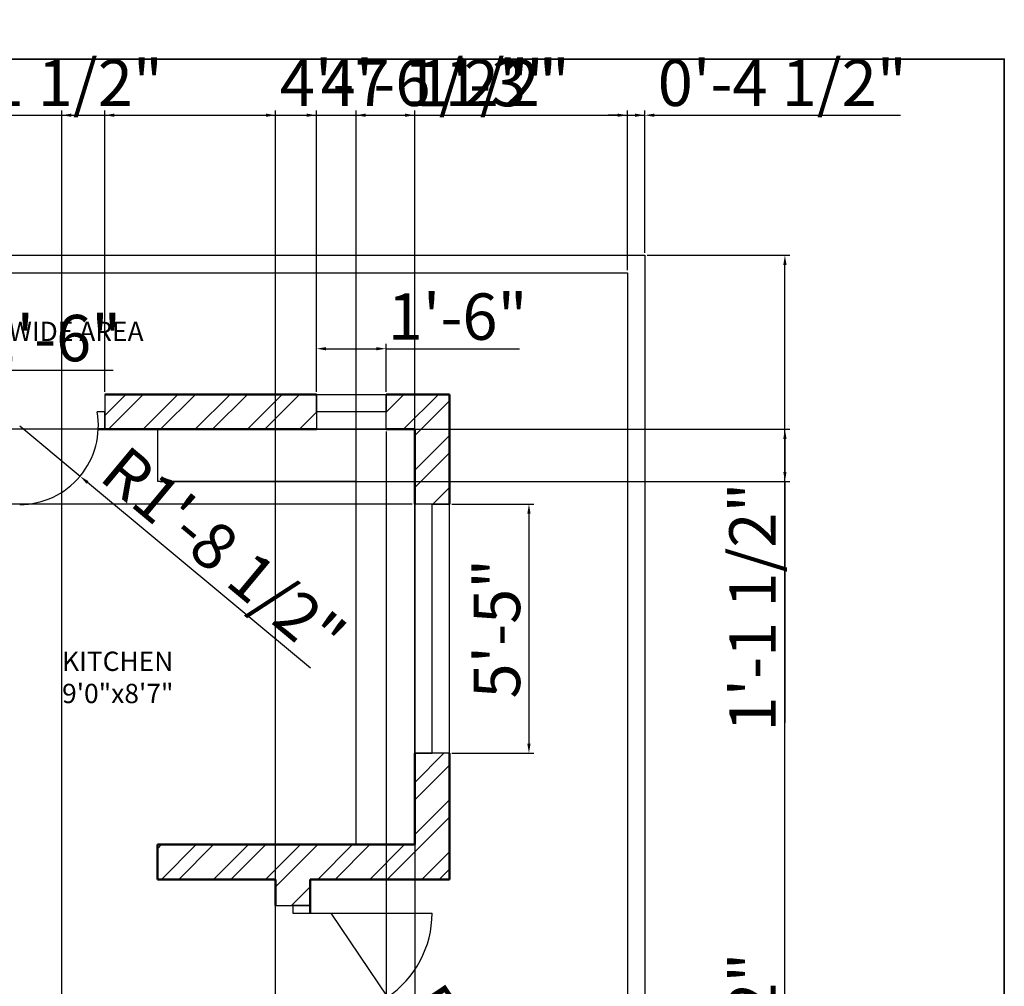
# Model space of a CAD drawing. Units: inches. Extents: x 1990 to 2869, y 1755 to 2533.
# Tile 6 of 6: x 2615 to 2869, y 2139 to 2389. Entities that reach past the tile are written whole.
import ezdxf

# ---------------------------------------------------------------- set-up
doc = ezdxf.new("R2010")
doc.units = ezdxf.units.IN
for name, color, linetype, lineweight in [('A-ANNO-DIMS', 171, 'Continuous', 18), ('A-ANNO-TTLB', 7, 'Continuous', 35), ('A-AREA-IDEN', 7, 'Continuous', 18), ('A-DOOR', 11, 'Continuous', 25), ('A-FLOR-CASE', 7, 'Continuous', 25), ('A-GLAZ', 121, 'Continuous', 25), ('A-WALL', 7, 'Continuous', 50), ('A-WALL-SITE', 7, 'Continuous', 30)]:
    doc.layers.add(name, color=color, linetype=linetype, lineweight=lineweight)
doc.layers.add('A-WALL-PATT', color=215, linetype='Continuous', lineweight=13, true_color=0xa953a0)
doc.styles.get("Standard").update_dxf_attribs({"font": 'arial.ttf'})
doc.dimstyles.new('ISO-25', dxfattribs={"dimtxt": 12, "dimasz": 2.5, "dimexe": 1.25, "dimexo": 0.625, "dimtad": 1, "dimdec": 0, "dimlunit": 3, "dimtxsty": 'Standard', "dimcen": 2.5, "dimadec": 0, "dimazin": 0, "dimtfac": 1, "dimtdec": 0, "dimtmove": 0, "dimatfit": 3, "dimfxl": 1, "dimarcsym": 0})

# ---------------------------------------------------------------- blocks, each defined once
blk = doc.blocks.new('*D11')
at = {"layer": 'A-ANNO-DIMS', "color": 0, "lineweight": -2, "transparency": 16777216}
for p, q in [((2726.6, 2263.68), (2747.77, 2263.68)), ((2746.52, 2261.18), (2746.52, 2201.68)), ((2726.6, 2199.18), (2747.77, 2199.18))]:
    blk.add_line(p, q, dxfattribs=at)
at = {"layer": 'A-ANNO-DIMS', "color": 0, "transparency": 16777216}
for points in [[(2746.1, 2261.18), (2746.94, 2261.18), (2746.52, 2263.68)], [(2746.1, 2201.68), (2746.94, 2201.68), (2746.52, 2199.18)]]:
    blk.add_solid(points, dxfattribs=at)
at = {"layer": 'Defpoints', "color": 0, "transparency": 16777216}
for p in [(2725.97, 2263.68), (2725.97, 2199.18), (2746.52, 2199.18)]:
    blk.add_point(p, dxfattribs=at)
at = {"layer": 'A-ANNO-DIMS', "color": 0, "transparency": 16777216, "insert": (2739.79, 2231.43), "char_height": 12, "attachment_point": 5, "rotation": 90}
blk.add_mtext('5\'-5"', dxfattribs=at)
blk = doc.blocks.new('*D12')
at = {"layer": 'A-ANNO-DIMS', "color": 0, "lineweight": -2, "transparency": 16777216}
for p, q in [((2691.55, 2292.68), (2691.55, 2305.13)), ((2709.55, 2292.68), (2709.55, 2305.13)), ((2694.05, 2303.88), (2707.05, 2303.88)), ((2709.55, 2303.88), (2744.07, 2303.88))]:
    blk.add_line(p, q, dxfattribs=at)
at = {"layer": 'A-ANNO-DIMS', "color": 0, "transparency": 16777216}
for points in [[(2694.05, 2304.29), (2694.05, 2303.46), (2691.55, 2303.88)], [(2707.05, 2304.29), (2707.05, 2303.46), (2709.55, 2303.88)]]:
    blk.add_solid(points, dxfattribs=at)
at = {"layer": 'Defpoints', "color": 0, "transparency": 16777216}
for p in [(2709.55, 2303.88), (2691.55, 2292.05), (2709.55, 2292.05)]:
    blk.add_point(p, dxfattribs=at)
at = {"layer": 'A-ANNO-DIMS', "color": 0, "transparency": 16777216, "insert": (2728.06, 2310.63), "char_height": 12, "attachment_point": 5}
blk.add_mtext('1\'-6"', dxfattribs=at)
blk = doc.blocks.new('*D13')
at = {"layer": 'A-ANNO-DIMS', "color": 0, "lineweight": -2, "transparency": 16777216}
for p, q in [((2586.47, 2292.68), (2586.47, 2299.57)), ((2604.47, 2292.68), (2604.47, 2299.57)), ((2588.97, 2298.32), (2601.97, 2298.32)), ((2604.47, 2298.32), (2638.99, 2298.32))]:
    blk.add_line(p, q, dxfattribs=at)
at = {"layer": 'A-ANNO-DIMS', "color": 0, "transparency": 16777216}
for points in [[(2588.97, 2298.74), (2588.97, 2297.9), (2586.47, 2298.32)], [(2601.97, 2298.74), (2601.97, 2297.9), (2604.47, 2298.32)]]:
    blk.add_solid(points, dxfattribs=at)
at = {"layer": 'Defpoints', "color": 0, "transparency": 16777216}
for p in [(2604.47, 2298.32), (2586.47, 2292.05), (2604.47, 2292.05)]:
    blk.add_point(p, dxfattribs=at)
at = {"layer": 'A-ANNO-DIMS', "color": 0, "transparency": 16777216, "insert": (2622.98, 2305.07), "char_height": 12, "attachment_point": 5}
blk.add_mtext('1\'-6"', dxfattribs=at)
blk = doc.blocks.new('WIN-64_5IN')
for p, q in [((0, 9), (0, 0)), ((0, 9), (64.5, 9)), ((64.5, 4.5), (64.5, 9)), ((64.5, 9), (64.5, 0)), ((0, 0), (0, 4.5)), ((0, 4.5), (64.5, 4.5)), ((64.5, 0), (0, 0))]:
    blk.add_line(p, q)
blk = doc.blocks.new('*D27')
at = {"layer": 'A-ANNO-DIMS', "color": 0, "lineweight": -2, "transparency": 16777216}
for p, q in [((2625.68, 1894.18), (2625.68, 2365.55)), ((2628.18, 2364.3), (2678.47, 2364.3)), ((2680.97, 1894.18), (2680.97, 2365.55)), ((2680.97, 2364.3), (2745.07, 2364.3))]:
    blk.add_line(p, q, dxfattribs=at)
at = {"layer": 'A-ANNO-DIMS', "color": 0, "transparency": 16777216}
for points in [[(2628.18, 2364.72), (2628.18, 2363.88), (2625.68, 2364.3)], [(2678.47, 2364.72), (2678.47, 2363.88), (2680.97, 2364.3)]]:
    blk.add_solid(points, dxfattribs=at)
at = {"layer": 'Defpoints', "color": 0, "transparency": 16777216}
for p in [(2680.97, 2364.3), (2625.68, 1893.55), (2680.97, 1893.55)]:
    blk.add_point(p, dxfattribs=at)
at = {"layer": 'A-ANNO-DIMS', "color": 0, "transparency": 16777216, "insert": (2714.27, 2371.13), "char_height": 12, "attachment_point": 5}
blk.add_mtext('4\'-7 1/2"', dxfattribs=at)
blk = doc.blocks.new('*D36')
at = {"layer": 'A-ANNO-DIMS', "color": 0, "lineweight": -2, "transparency": 16777216}
for p, q in [((2716.35, 2283.05), (2016.97, 2283.05)), ((2018.22, 2280.55), (2018.22, 2266.18)), ((2716.35, 2263.68), (2016.97, 2263.68)), ((2018.22, 2263.68), (2018.22, 2201.19))]:
    blk.add_line(p, q, dxfattribs=at)
at = {"layer": 'A-ANNO-DIMS', "color": 0, "transparency": 16777216}
for points in [[(2017.8, 2280.55), (2018.64, 2280.55), (2018.22, 2283.05)], [(2017.8, 2266.18), (2018.64, 2266.18), (2018.22, 2263.68)]]:
    blk.add_solid(points, dxfattribs=at)
at = {"layer": 'Defpoints', "color": 0, "transparency": 16777216}
for p in [(2716.97, 2283.05), (2018.22, 2263.68), (2716.97, 2263.68)]:
    blk.add_point(p, dxfattribs=at)
at = {"layer": 'A-ANNO-DIMS', "color": 0, "transparency": 16777216, "insert": (2011.39, 2231.19), "char_height": 12, "attachment_point": 5, "rotation": 90}
blk.add_mtext('1\'-7 1/2"', dxfattribs=at)
blk = doc.blocks.new('*D38')
at = {"layer": 'A-ANNO-DIMS', "color": 0, "lineweight": -2, "transparency": 16777216}
for p, q in [((2560.97, 2292.68), (2560.97, 2365.55)), ((2563.47, 2364.3), (2583.97, 2364.3)), ((2586.47, 2292.68), (2586.47, 2365.55)), ((2586.47, 2364.3), (2650.29, 2364.3))]:
    blk.add_line(p, q, dxfattribs=at)
at = {"layer": 'A-ANNO-DIMS', "color": 0, "transparency": 16777216}
for points in [[(2563.47, 2364.72), (2563.47, 2363.88), (2560.97, 2364.3)], [(2583.97, 2364.72), (2583.97, 2363.88), (2586.47, 2364.3)]]:
    blk.add_solid(points, dxfattribs=at)
at = {"layer": 'Defpoints', "color": 0, "transparency": 16777216}
for p in [(2586.47, 2364.3), (2560.97, 2292.05), (2586.47, 2292.05)]:
    blk.add_point(p, dxfattribs=at)
at = {"layer": 'A-ANNO-DIMS', "color": 0, "transparency": 16777216, "insert": (2619.63, 2371.13), "char_height": 12, "attachment_point": 5}
blk.add_mtext('2\'-1 1/2"', dxfattribs=at)
blk = doc.blocks.new('*D39')
at = {"layer": 'A-ANNO-DIMS', "color": 0, "lineweight": -2, "transparency": 16777216}
for p, q in [((2709.55, 2282.43), (2709.55, 1764.83)), ((2716.97, 2282.43), (2716.97, 1764.83)), ((2712.05, 1766.08), (2714.47, 1766.08)), ((2716.97, 1766.08), (2780.58, 1766.08))]:
    blk.add_line(p, q, dxfattribs=at)
at = {"layer": 'A-ANNO-DIMS', "color": 0, "transparency": 16777216}
for points in [[(2712.05, 1766.49), (2712.05, 1765.66), (2709.55, 1766.08)], [(2714.47, 1766.49), (2714.47, 1765.66), (2716.97, 1766.08)]]:
    blk.add_solid(points, dxfattribs=at)
at = {"layer": 'Defpoints', "color": 0, "transparency": 16777216}
for p in [(2709.55, 2283.05), (2716.97, 2283.05), (2716.97, 1766.08)]:
    blk.add_point(p, dxfattribs=at)
at = {"layer": 'A-ANNO-DIMS', "color": 0, "transparency": 16777216, "insert": (2750.03, 1772.91), "char_height": 12, "attachment_point": 5}
blk.add_mtext('0\'-7 1/2"', dxfattribs=at)
blk = doc.blocks.new('*D43')
at = {"layer": 'A-ANNO-DIMS', "color": 0, "lineweight": -2, "transparency": 16777216}
for p, q in [((2651.18, 2283.05), (2813.97, 2283.05)), ((2812.72, 2280.55), (2812.72, 2272.01)), ((2651.18, 2269.51), (2813.97, 2269.51)), ((2812.72, 2269.51), (2812.72, 2207.03))]:
    blk.add_line(p, q, dxfattribs=at)
at = {"layer": 'A-ANNO-DIMS', "color": 0, "transparency": 16777216}
for points in [[(2812.3, 2280.55), (2813.14, 2280.55), (2812.72, 2283.05)], [(2812.3, 2272.01), (2813.14, 2272.01), (2812.72, 2269.51)]]:
    blk.add_solid(points, dxfattribs=at)
at = {"layer": 'Defpoints', "color": 0, "transparency": 16777216}
for p in [(2650.55, 2283.05), (2650.55, 2269.51), (2812.72, 2269.51)]:
    blk.add_point(p, dxfattribs=at)
at = {"layer": 'A-ANNO-DIMS', "color": 0, "transparency": 16777216, "insert": (2805.89, 2237.02), "char_height": 12, "attachment_point": 5, "rotation": 90}
blk.add_mtext('1\'-1 1/2"', dxfattribs=at)
blk = doc.blocks.new('*D44')
at = {"layer": 'A-ANNO-DIMS', "color": 0, "lineweight": -2, "transparency": 16777216}
for p, q in [((2701.8, 2176.18), (2701.8, 2365.55)), ((2704.3, 2364.3), (2714.47, 2364.3)), ((2716.97, 2176.18), (2716.97, 2365.55)), ((2716.97, 2364.3), (2751.49, 2364.3))]:
    blk.add_line(p, q, dxfattribs=at)
at = {"layer": 'A-ANNO-DIMS', "color": 0, "transparency": 16777216}
for points in [[(2704.3, 2364.72), (2704.3, 2363.88), (2701.8, 2364.3)], [(2714.47, 2364.72), (2714.47, 2363.88), (2716.97, 2364.3)]]:
    blk.add_solid(points, dxfattribs=at)
at = {"layer": 'Defpoints', "color": 0, "transparency": 16777216}
for p in [(2716.97, 2364.3), (2701.8, 2175.55), (2716.97, 2175.55)]:
    blk.add_point(p, dxfattribs=at)
at = {"layer": 'A-ANNO-DIMS', "color": 0, "transparency": 16777216, "insert": (2735.48, 2371.06), "char_height": 12, "attachment_point": 5}
blk.add_mtext('1\'-3"', dxfattribs=at)
blk = doc.blocks.new('*D46')
at = {"layer": 'A-ANNO-DIMS', "color": 0, "lineweight": -2, "transparency": 16777216}
for p, q in [((2636.82, 2292.68), (2636.82, 2365.55)), ((2639.32, 2364.3), (2689.05, 2364.3)), ((2691.55, 2292.68), (2691.55, 2365.55)), ((2691.55, 2364.3), (2755.64, 2364.3))]:
    blk.add_line(p, q, dxfattribs=at)
at = {"layer": 'A-ANNO-DIMS', "color": 0, "transparency": 16777216}
for points in [[(2639.32, 2364.72), (2639.32, 2363.88), (2636.82, 2364.3)], [(2689.05, 2364.72), (2689.05, 2363.88), (2691.55, 2364.3)]]:
    blk.add_solid(points, dxfattribs=at)
at = {"layer": 'Defpoints', "color": 0, "transparency": 16777216}
for p in [(2691.55, 2364.3), (2636.82, 2292.05), (2691.55, 2292.05)]:
    blk.add_point(p, dxfattribs=at)
at = {"layer": 'A-ANNO-DIMS', "color": 0, "transparency": 16777216, "insert": (2724.85, 2371.13), "char_height": 12, "attachment_point": 5}
blk.add_mtext('4\'-6 1/2"', dxfattribs=at)
blk = doc.blocks.new('*D47')
at = {"layer": 'A-ANNO-DIMS', "color": 0, "lineweight": -2, "transparency": 16777216}
for p, q in [((2769.47, 2364.3), (2766.97, 2364.3)), ((2771.97, 2324.18), (2771.97, 2365.55)), ((2771.97, 2364.3), (2776.47, 2364.3)), ((2776.47, 2328.68), (2776.47, 2365.55)), ((2778.97, 2364.3), (2842.58, 2364.3))]:
    blk.add_line(p, q, dxfattribs=at)
at = {"layer": 'A-ANNO-DIMS', "color": 0, "transparency": 16777216}
for points in [[(2769.47, 2364.72), (2769.47, 2363.88), (2771.97, 2364.3)], [(2778.97, 2364.72), (2778.97, 2363.88), (2776.47, 2364.3)]]:
    blk.add_solid(points, dxfattribs=at)
at = {"layer": 'Defpoints', "color": 0, "transparency": 16777216}
for p in [(2776.47, 2364.3), (2776.47, 2328.05), (2771.97, 2323.55)]:
    blk.add_point(p, dxfattribs=at)
at = {"layer": 'A-ANNO-DIMS', "color": 0, "transparency": 16777216, "insert": (2812.03, 2371.13), "char_height": 12, "attachment_point": 5}
blk.add_mtext('0\'-4 1/2"', dxfattribs=at)
blk = doc.blocks.new('*D48')
at = {"layer": 'A-ANNO-DIMS', "color": 0, "lineweight": -2, "transparency": 16777216}
for p, q in [((2054.47, 2328.68), (2054.47, 2365.55)), ((2056.97, 2364.3), (2773.97, 2364.3)), ((2776.47, 2328.68), (2776.47, 2365.55))]:
    blk.add_line(p, q, dxfattribs=at)
at = {"layer": 'A-ANNO-DIMS', "color": 0, "transparency": 16777216}
for points in [[(2056.97, 2364.72), (2056.97, 2363.88), (2054.47, 2364.3)], [(2773.97, 2364.72), (2773.97, 2363.88), (2776.47, 2364.3)]]:
    blk.add_solid(points, dxfattribs=at)
at = {"layer": 'Defpoints', "color": 0, "transparency": 16777216}
for p in [(2776.47, 2364.3), (2054.47, 2328.05), (2776.47, 2328.05)]:
    blk.add_point(p, dxfattribs=at)
at = {"layer": 'A-ANNO-DIMS', "color": 0, "transparency": 16777216, "insert": (2415.47, 2371.05), "char_height": 12, "attachment_point": 5}
blk.add_mtext('60\'-2"', dxfattribs=at)
blk = doc.blocks.new('*D49')
at = {"layer": 'A-ANNO-DIMS', "color": 0, "lineweight": -2, "transparency": 16777216}
for p, q in [((2777.1, 2328.05), (2813.97, 2328.05)), ((2812.72, 1887.05), (2812.72, 2325.55)), ((2777.1, 1884.55), (2813.97, 1884.55))]:
    blk.add_line(p, q, dxfattribs=at)
at = {"layer": 'A-ANNO-DIMS', "color": 0, "transparency": 16777216}
for points in [[(2812.3, 2325.55), (2813.14, 2325.55), (2812.72, 2328.05)], [(2812.3, 1887.05), (2813.14, 1887.05), (2812.72, 1884.55)]]:
    blk.add_solid(points, dxfattribs=at)
at = {"layer": 'Defpoints', "color": 0, "transparency": 16777216}
for p in [(2776.47, 2328.05), (2812.72, 2328.05), (2776.47, 1884.55)]:
    blk.add_point(p, dxfattribs=at)
at = {"layer": 'A-ANNO-DIMS', "color": 0, "transparency": 16777216, "insert": (2805.89, 2106.3), "char_height": 12, "attachment_point": 5, "rotation": 90}
blk.add_mtext('36\'-11 1/2"', dxfattribs=at)
blk = doc.blocks.new('*D51')
at = {"layer": 'A-ANNO-DIMS', "color": 0, "lineweight": -2, "transparency": 16777216}
for p, q in [((2695.32, 2157.77), (2709.92, 2136.08)), ((2737.62, 2094.9), (2711.31, 2134))]:
    blk.add_line(p, q, dxfattribs=at)
at = {"layer": 'A-ANNO-DIMS', "color": 0, "transparency": 16777216}
blk.add_solid([(2711.66, 2134.24), (2710.97, 2133.77), (2709.92, 2136.08)], dxfattribs=at)
at = {"layer": 'Defpoints', "color": 0, "transparency": 16777216}
for p in [(2695.32, 2157.77), (2709.92, 2136.08)]:
    blk.add_point(p, dxfattribs=at)
at = {"layer": 'A-ANNO-DIMS', "color": 0, "transparency": 16777216, "insert": (2730.68, 2117.12), "char_height": 12, "attachment_point": 5, "rotation": 303.9296}
blk.add_mtext('R2\'-2"', dxfattribs=at)
blk = doc.blocks.new('*D59')
at = {"layer": 'A-ANNO-DIMS', "color": 0, "lineweight": -2, "transparency": 16777216}
for p, q in [((2614.81, 2283.89), (2630.43, 2270.87)), ((2690.03, 2221.18), (2632.35, 2269.27))]:
    blk.add_line(p, q, dxfattribs=at)
at = {"layer": 'A-ANNO-DIMS', "color": 0, "transparency": 16777216}
blk.add_solid([(2632.62, 2269.59), (2632.09, 2268.95), (2630.43, 2270.87)], dxfattribs=at)
at = {"layer": 'Defpoints', "color": 0, "transparency": 16777216}
for p in [(2614.81, 2283.89), (2630.43, 2270.87)]:
    blk.add_point(p, dxfattribs=at)
at = {"layer": 'A-ANNO-DIMS', "color": 0, "transparency": 16777216, "insert": (2666.52, 2249.67), "char_height": 12, "attachment_point": 5, "rotation": 320.1799}
blk.add_mtext('R1\'-8 1/2"', dxfattribs=at)

msp = doc.modelspace()

# ---------------------------------------------------------------- hatches: boundary and pattern name
at = {"layer": 'A-WALL-PATT'}
h = msp.add_hatch(dxfattribs=at)
h.set_pattern_fill('ANSI32', color=256)
h.paths.add_polyline_path([(2193.46, 2287.55), (2131.97, 2287.55), (2131.97, 2278.55), (2193.46, 2278.55)])
h.paths.add_polyline_path([(2113.97, 2278.55), (2113.97, 2287.55), (2104.97, 2287.55), (2104.97, 2257.5), (2113.97, 2257.5)])
h.paths.add_polyline_path([(2113.97, 2205), (2104.97, 2205), (2104.97, 2166.55), (2140.97, 2166.55), (2140.97, 2160.48), (2149.97, 2160.48), (2149.97, 2166.55), (2170.14, 2166.55), (2170.14, 2175.55), (2113.97, 2175.55)])
h.paths.add_polyline_path([(2278.97, 2287.55), (2244.47, 2287.55), (2244.47, 2278.55), (2274.47, 2278.55), (2274.47, 2200.55), (2226.47, 2200.55), (2226.47, 2219.37), (2221.97, 2219.37), (2221.97, 2175.55), (2221.97, 2166.55), (2226.47, 2166.55), (2226.47, 2196.05), (2274.47, 2196.05), (2274.47, 2166.55), (2284.01, 2166.55), (2284.01, 2171.05), (2284.01, 2175.55), (2278.97, 2175.55), (2278.97, 2278.55)])
h.paths.add_polyline_path([(2226.47, 2283.05), (2226.47, 2287.55), (2217.66, 2287.55), (2217.66, 2283.05), (2217.66, 2278.55), (2221.97, 2278.55), (2221.97, 2255.21), (2226.47, 2255.21), (2226.47, 2278.55)])
h.paths.add_polyline_path([(2560.97, 2328.05), (2551.97, 2328.05), (2269.97, 2328.05), (2269.97, 2319.05), (2278.97, 2319.05), (2410.97, 2319.05), (2410.97, 2187.05), (2346.47, 2187.05), (2346.47, 2175.55), (2319.77, 2175.55), (2319.77, 2166.55), (2346.47, 2166.55), (2346.47, 2128.22), (2350.97, 2128.22), (2350.97, 2178.05), (2410.97, 2178.05), (2410.97, 2175.55), (2410.97, 2106.05), (2350.97, 2106.05), (2350.97, 2108.72), (2348.72, 2108.72), (2346.47, 2108.72), (2346.47, 2106.05), (2342.3, 2106.05), (2342.3, 2097.05), (2346.47, 2097.05), (2350.97, 2097.05), (2410.97, 2097.05), (2410.97, 1974.05), (2373.73, 1974.05), (2373.73, 1965.05), (2419.97, 1965.05), (2447.99, 1965.05), (2447.99, 1969.55), (2447.99, 1974.05), (2419.97, 1974.05), (2419.97, 2097.05), (2484.47, 2097.05), (2489.55, 2097.05), (2489.55, 2106.05), (2484.47, 2106.05), (2484.47, 2108.84), (2482.22, 2108.84), (2479.97, 2108.84), (2479.97, 2106.05), (2419.97, 2106.05), (2419.97, 2175.55), (2419.97, 2178.05), (2479.97, 2178.05), (2479.97, 2128.49), (2484.47, 2128.49), (2484.47, 2166.55), (2511.88, 2166.55), (2511.88, 2171.05), (2511.88, 2175.55), (2484.47, 2175.55), (2484.47, 2187.05), (2479.97, 2187.05), (2419.97, 2187.05), (2419.97, 2319.05), (2551.97, 2319.05), (2560.97, 2319.05)])
h.paths.add_polyline_path([(2586.47, 2292.05), (2560.97, 2292.05), (2551.97, 2292.05), (2551.97, 2175.55), (2547.37, 2175.55), (2547.37, 2166.55), (2556.47, 2166.55), (2556.47, 2175.55), (2556.47, 2205.05), (2604.47, 2205.05), (2604.47, 2166.55), (2608.97, 2166.55), (2608.97, 2175.55), (2608.97, 2205.05), (2608.97, 2228.1), (2604.47, 2228.1), (2604.47, 2209.55), (2556.47, 2209.55), (2556.47, 2283.05), (2586.47, 2283.05)])
h.paths.add_polyline_path([(2691.55, 2292.05), (2690.86, 2292.05), (2636.82, 2292.05), (2636.82, 2283.05), (2691.55, 2283.05)])
h.paths.add_polyline_path([(2725.97, 2292.05), (2716.97, 2292.05), (2709.55, 2292.05), (2709.55, 2287.55), (2709.55, 2283.05), (2716.97, 2283.05), (2716.97, 2263.68), (2725.97, 2263.68)])
h.paths.add_polyline_path([(2725.97, 2199.18), (2716.97, 2199.18), (2716.97, 2180.05), (2716.97, 2175.55), (2650.43, 2175.55), (2650.43, 2166.55), (2680.97, 2166.55), (2680.97, 2159.77), (2689.97, 2159.77), (2689.97, 2166.55), (2725.97, 2166.55)])
h.paths.add_polyline_path([(2536.97, 2061.55), (2554.82, 2061.55), (2554.82, 2070.55), (2536.97, 2070.55), (2536.97, 2097.05), (2536.97, 2106.05), (2524.42, 2106.05), (2524.42, 2101.55), (2524.42, 2097.05), (2527.97, 2097.05), (2527.97, 1974.05), (2497.49, 1974.05), (2497.49, 1965.05), (2527.97, 1965.05), (2527.97, 1929.96), (2536.97, 1929.96)])
h.paths.add_polyline_path([(2689.97, 1945.55), (2685.47, 1945.55), (2680.97, 1945.55), (2680.97, 1893.55), (2625.68, 1893.55), (2625.68, 1884.55), (2689.97, 1884.55), (2689.97, 1893.55)])
h.paths.add_polyline_path([(2168.89, 2070.55), (2149.97, 2070.55), (2149.97, 2116.52), (2145.47, 2116.52), (2140.97, 2116.52), (2140.97, 1977.7), (2145.47, 1977.7), (2145.47, 1977.63), (2149.97, 1977.55), (2149.97, 2061.55), (2168.89, 2061.55)])
h.paths.add_polyline_path([(2302.97, 2097.05), (2306.2, 2097.05), (2306.2, 2106.05), (2293.97, 2106.05), (2293.97, 2097.05), (2293.97, 2070.55), (2269.93, 2070.55), (2269.93, 2061.55), (2293.97, 2061.55), (2293.97, 1930.78), (2302.97, 1930.78), (2302.97, 1965.05), (2324.23, 1965.05), (2324.23, 1969.55), (2324.23, 1974.05), (2302.97, 1974.05)])
h.paths.add_polyline_path([(2149.97, 1928.2), (2145.47, 1928.2), (2140.97, 1928.2), (2140.97, 1889.05), (2140.97, 1884.55), (2178.84, 1884.55), (2178.84, 1889.05), (2178.84, 1893.55), (2149.97, 1893.55)])
h.paths.add_polyline_path([(2302.97, 1898.24), (2298.47, 1898.24), (2293.97, 1898.24), (2293.97, 1893.55), (2243.34, 1893.55), (2243.34, 1884.55), (2302.97, 1884.55)])

# ---------------------------------------------------------------- linework, layer by layer
at = {"layer": 'A-ANNO-TTLB'}
msp.add_lwpolyline([(1989.71, 2378.83), (2869.46, 2378.83), (2869.46, 1755.45), (1989.71, 1755.45)], close=True, dxfattribs=at)
at = {"layer": 'A-DOOR'}
for p, q in [((2636.82, 2292.05), (2636.82, 2283.05)), ((2636.82, 2287.55), (2634.82, 2287.55)), ((2636.82, 2283.05), (2636.82, 2287.55)), ((2680.97, 2159.77), (2689.97, 2159.77)), ((2689.97, 2159.77), (2685.47, 2159.77)), ((2685.47, 2159.77), (2685.47, 2157.77)), ((2685.47, 2157.77), (2721.47, 2157.77))]:
    msp.add_line(p, q, dxfattribs=at)
for centre, radius, start, end in [((2614.81, 2283.89), 20.34, 270, 10.3586), ((2695.32, 2157.77), 26.15, 247.8615, 0)]:
    msp.add_arc(centre, radius, start, end, dxfattribs=at)
at = {"layer": 'A-FLOR-CASE'}
for p, q in [((2650.55, 2269.51), (2650.55, 2283.05)), ((2701.8, 2269.51), (2650.55, 2269.51)), ((2701.8, 2175.55), (2701.8, 2269.51))]:
    msp.add_line(p, q, dxfattribs=at)
at = {"layer": 'A-GLAZ'}
for p, q in [((2690.86, 2292.05), (2709.55, 2292.05)), ((2691.55, 2287.55), (2691.55, 2292.05)), ((2691.55, 2292.05), (2691.55, 2283.05)), ((2709.55, 2283.05), (2709.55, 2292.05)), ((2709.55, 2292.05), (2709.55, 2287.55)), ((2709.55, 2287.55), (2691.55, 2287.55)), ((2709.55, 2283.05), (2691.55, 2283.05))]:
    msp.add_line(p, q, dxfattribs=at)
at = {"layer": 'A-WALL'}
for p, q in [((2636.82, 2292.05), (2691.55, 2292.05)), ((2709.55, 2292.05), (2716.97, 2292.05)), ((2716.97, 2292.05), (2725.97, 2292.05)), ((2725.97, 2292.05), (2725.97, 2263.68)), ((2635.13, 2283.05), (2691.55, 2283.05)), ((2709.55, 2283.05), (2716.97, 2283.05)), ((2716.97, 2283.05), (2716.97, 2263.68)), ((2716.97, 2199.18), (2716.97, 2180.05)), ((2725.97, 2199.18), (2725.97, 2166.55)), ((2716.97, 2175.55), (2716.97, 2180.05)), ((2650.43, 2175.55), (2716.97, 2175.55)), ((2650.43, 2175.55), (2650.43, 2166.55)), ((2680.97, 2166.55), (2650.43, 2166.55)), ((2680.97, 2166.55), (2680.97, 2159.77)), ((2725.97, 2166.55), (2689.97, 2166.55)), ((2689.97, 2166.55), (2689.97, 2157.77))]:
    msp.add_line(p, q, dxfattribs=at)
at = {"layer": 'A-WALL-SITE'}
for p, q in [((2054.47, 2328.05), (2776.47, 2328.05)), ((2776.47, 2328.05), (2776.47, 1884.55)), ((2560.97, 2323.55), (2771.97, 2323.55)), ((2771.97, 2323.55), (2771.97, 1884.55))]:
    msp.add_line(p, q, dxfattribs=at)

# ---------------------------------------------------------------- block references
at = {"layer": 'A-GLAZ', "extrusion": (0, 0, -1), "zscale": -1, "rotation": 90}
msp.add_blockref('WIN-64_5IN', (-2716.97, 2199.18), dxfattribs=at)

# ---------------------------------------------------------------- texts
at = {"layer": 'A-AREA-IDEN', "char_height": 5, "attachment_point": 1}
for s, width, insert in [('3\'0" WIDE AREA', 91.327, (2597.75, 2310.86)), ('KITCHEN\\P9\'0"x8\'7"', 224.984, (2625.77, 2225.49))]:
    msp.add_mtext_dynamic_manual_height_columns(s, width=width, gutter_width=12.5, heights=[0], dxfattribs=dict(at, insert=insert))

# ---------------------------------------------------------------- dimensions: what is measured, and where the dimension line sits
at = {"layer": 'A-ANNO-DIMS'}
for base, p1, p2, override, picture, middle in [((2586.47, 2364.3), (2560.97, 2292.05), (2586.47, 2292.05), {"dimdec": 1, "dimlfac": 1, "dimrnd": 0, "dimzin": 1, "dimdsep": 46, "dimlunit": 4, "dimfrac": 2}, '*D38', (2619.63, 2371.13)), ((2680.97, 2364.3), (2625.68, 1893.55), (2680.97, 1893.55), {"dimdec": 1, "dimlfac": 1, "dimrnd": 0, "dimzin": 1, "dimdsep": 46, "dimlunit": 4, "dimfrac": 2}, '*D27', (2714.27, 2371.13)), ((2691.55, 2364.3), (2636.82, 2292.05), (2691.55, 2292.05), {"dimdec": 1, "dimlfac": 1, "dimrnd": 0, "dimzin": 1, "dimdsep": 46, "dimlunit": 4, "dimfrac": 2}, '*D46', (2724.85, 2371.13)), ((2776.47, 2364.3), (2771.97, 2323.55), (2776.47, 2328.05), {"dimdec": 1, "dimlfac": 1, "dimrnd": 0, "dimzin": 1, "dimdsep": 46, "dimlunit": 4, "dimfrac": 2}, '*D47', (2812.03, 2371.13)), ((2776.47, 2364.3), (2054.47, 2328.05), (2776.47, 2328.05), {"dimdec": 1, "dimlfac": 1, "dimrnd": 0, "dimzin": 1, "dimdsep": 46, "dimlunit": 4, "dimfrac": 2}, '*D48', (2415.47, 2371.05)), ((2716.97, 2364.3), (2701.8, 2175.55), (2716.97, 2175.55), {"dimdec": 1, "dimlfac": 1, "dimrnd": 0, "dimzin": 1, "dimdsep": 46, "dimlunit": 4, "dimfrac": 2}, '*D44', (2735.48, 2371.06)), ((2709.55, 2303.88), (2691.55, 2292.05), (2709.55, 2292.05), {"dimclrd": 0, "dimclre": 0, "dimclrt": 0}, '*D12', (2728.06, 2310.63)), ((2604.47, 2298.32), (2586.47, 2292.05), (2604.47, 2292.05), {"dimclrd": 0, "dimclre": 0, "dimclrt": 0}, '*D13', (2622.98, 2305.07)), ((2716.97, 1766.08), (2709.55, 2283.05), (2716.97, 2283.05), {"dimdec": 1, "dimlfac": 1, "dimrnd": 0, "dimzin": 1, "dimdsep": 46, "dimlunit": 4, "dimfrac": 2}, '*D39', (2750.03, 1772.91))]:
    dim = msp.add_linear_dim(base=base, p1=p1, p2=p2, dimstyle='ISO-25', override=override, dxfattribs=at)
    dim.commit()
    dim.dimension.update_dxf_attribs({"geometry": picture, "text_midpoint": middle})
for base, p1, p2, override, picture, middle in [((2812.72, 2328.05), (2776.47, 1884.55), (2776.47, 2328.05), {"dimdec": 1, "dimlfac": 1, "dimrnd": 0, "dimzin": 1, "dimdsep": 46, "dimlunit": 4, "dimfrac": 2}, '*D49', (2805.89, 2106.3)), ((2018.22, 2263.68), (2716.97, 2283.05), (2716.97, 2263.68), {"dimdec": 1, "dimlfac": 1, "dimrnd": 0, "dimzin": 1, "dimdsep": 46, "dimlunit": 4, "dimfrac": 2}, '*D36', (2011.39, 2231.19)), ((2812.72, 2269.51), (2650.55, 2283.05), (2650.55, 2269.51), {"dimdec": 1, "dimlfac": 1, "dimrnd": 0, "dimzin": 1, "dimdsep": 46, "dimlunit": 4, "dimfrac": 2}, '*D43', (2805.89, 2237.02)), ((2746.51856684, 2199.17564348), (2725.97134122, 2263.67564348), (2725.97134122, 2199.17564348), {"dimclrd": 0, "dimclre": 0, "dimclrt": 0}, '*D11', (2739.79124761, 2231.42564348))]:
    dim = msp.add_linear_dim(base=base, p1=p1, p2=p2, angle=90, dimstyle='ISO-25', override=override, dxfattribs=at)
    dim.commit()
    dim.dimension.update_dxf_attribs({"geometry": picture, "text_midpoint": middle})
for center, mpoint, picture, middle in [((2614.81, 2283.89), (2630.43, 2270.87), '*D59', (2666.52, 2249.67)), ((2695.32, 2157.77), (2709.92, 2136.08), '*D51', (2730.68, 2117.12))]:
    dim = msp.add_radius_dim(center=center, mpoint=mpoint, dimstyle='ISO-25', override={"dimdec": 1, "dimlfac": 1, "dimrnd": 0, "dimzin": 1, "dimdsep": 46, "dimlunit": 4, "dimfrac": 2}, dxfattribs=at)
    dim.commit()
    dim.dimension.update_dxf_attribs({"geometry": picture, "text_midpoint": middle})

doc.saveas('drawing.dxf')
